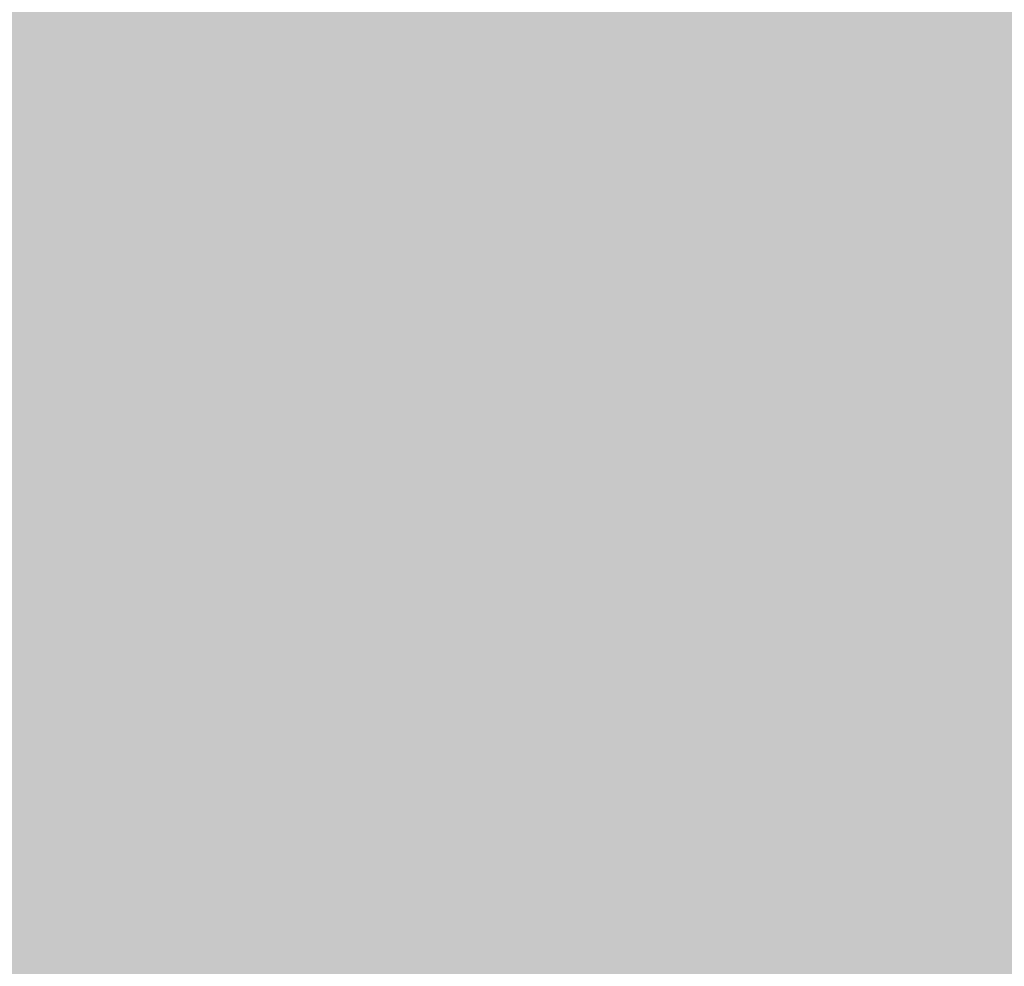
# Model space of a CAD drawing. Units: inches. Extents: x 2083 to 3317, y 1141 to 2115.
# Tile 132 of 256: x 3119.674 to 3123.979, y 1267.234 to 1271.372. Entities that reach past the tile are written whole.
import ezdxf

# ---------------------------------------------------------------- set-up
doc = ezdxf.new("R2010")
doc.units = ezdxf.units.IN
doc.layers.add('A-ANNO-DIMS', color=2, linetype='Continuous', lineweight=18)
doc.layers.add('A-WALL-PATT', color=251, linetype='Continuous', lineweight=13, true_color=0x636466)
doc.styles.get("Standard").update_dxf_attribs({"font": 'arial.ttf'})
doc.dimstyles.new('ISO-25', dxfattribs={"dimtxt": 12, "dimasz": 12, "dimexe": 1.25, "dimexo": 0.625, "dimtad": 1, "dimlunit": 3, "dimtxsty": 'Standard', "dimcen": 2.5, "dimadec": 0, "dimazin": 0, "dimtfac": 1, "dimtmove": 0, "dimatfit": 3, "dimfxl": 1, "dimarcsym": 0})

# ---------------------------------------------------------------- blocks, each defined once
blk = doc.blocks.new('*D26')
at = {"layer": 'A-ANNO-DIMS', "color": 0, "lineweight": -2, "transparency": 16777216}
for p, q in [((3088.9858, 1274.9151), (3088.9858, 1270.952)), ((3111.24, 1274.9151), (3111.24, 1270.952)), ((3076.9858, 1272.202), (2840.2624, 1272.202)), ((3111.24, 1272.202), (3088.9858, 1272.202)), ((3123.24, 1272.202), (3135.24, 1272.202))]:
    blk.add_line(p, q, dxfattribs=at)
at = {"layer": 'A-ANNO-DIMS', "color": 0, "transparency": 16777216}
for points in [[(3076.9858, 1274.202), (3076.9858, 1270.202), (3088.9858, 1272.202)], [(3123.24, 1274.202), (3123.24, 1270.202), (3111.24, 1272.202)]]:
    blk.add_solid(points, dxfattribs=at)
at = {"layer": 'Defpoints', "color": 0, "transparency": 16777216}
for p in [(3088.9858, 1275.5401), (3111.24, 1275.5401), (3088.9858, 1272.202)]:
    blk.add_point(p, dxfattribs=at)
at = {"layer": 'A-ANNO-DIMS', "color": 0, "transparency": 16777216, "insert": (2952.6241, 1279.0316), "char_height": 12, "attachment_point": 5}
blk.add_mtext('NIGHTSTAND 1\'-10 1/2" TYP.', dxfattribs=at)
blk = doc.blocks.new('*D27')
at = {"layer": 'A-ANNO-DIMS', "color": 0, "lineweight": -2, "transparency": 16777216}
for p, q in [((3114.5782, 1309.7943), (3114.5782, 1321.7943)), ((3111.865, 1297.7943), (3115.8282, 1297.7943)), ((3114.5782, 1297.7943), (3114.5782, 1275.5401)), ((3111.865, 1275.5401), (3115.8282, 1275.5401)), ((3114.5782, 1263.5401), (3114.5782, 1140.9886))]:
    blk.add_line(p, q, dxfattribs=at)
at = {"layer": 'A-ANNO-DIMS', "color": 0, "transparency": 16777216}
for points in [[(3112.5782, 1309.7943), (3116.5782, 1309.7943), (3114.5782, 1297.7943)], [(3112.5782, 1263.5401), (3116.5782, 1263.5401), (3114.5782, 1275.5401)]]:
    blk.add_solid(points, dxfattribs=at)
at = {"layer": 'Defpoints', "color": 0, "transparency": 16777216}
for p in [(3111.24, 1297.7943), (3111.24, 1275.5401), (3114.5782, 1275.5401)]:
    blk.add_point(p, dxfattribs=at)
at = {"layer": 'A-ANNO-DIMS', "color": 0, "transparency": 16777216, "insert": (3107.7485, 1196.2643), "char_height": 12, "attachment_point": 5, "rotation": 90}
blk.add_mtext('1\'-10 1/2" TYP.', dxfattribs=at)

msp = doc.modelspace()

# ---------------------------------------------------------------- hatches: boundary and pattern name
at = {"layer": 'A-WALL-PATT'}
h = msp.add_hatch(color=256, dxfattribs=at)
h.dxf.hatch_style = 1
h.paths.add_polyline_path([(3126.9598, 2020.7614), (2748.9598, 2020.7614), (2604.9598, 2020.7614), (2226.9598, 2020.7614), (2226.9598, 1702.7614), (2466.9598, 1702.7614), (2466.9598, 1582.7614), (2418.9598, 1582.7614), (2418.9598, 1477.7614), (2226.9598, 1477.7614), (2226.9598, 1263.2614), (2544.9598, 1263.2614), (2544.9598, 1411.7614), (2604.9598, 1411.7614), (2685.9598, 1411.7614), (2685.9598, 1420.7614), (2604.9598, 1420.7614), (2604.9598, 1573.7614), (2604.9598, 1702.7614), (2604.9598, 2011.7614), (2748.9598, 2011.7614), (2748.9598, 1702.7614), (2862.9598, 1702.7614), (2862.9598, 1621.7614), (2871.9598, 1621.7614), (2871.9598, 1702.7614), (2883.9598, 1702.7614), (2883.9598, 1706.9395, -0.026459), (2883.9598, 1711.7614), (2757.9598, 1711.7614), (2757.9598, 1807.7614), (2787.9598, 1807.7614), (2787.9598, 1812.2614), (2757.9598, 1812.2614), (2757.9598, 2011.7614), (2877.9598, 2011.7614), (2877.9598, 1812.2614), (2847.9598, 1812.2614), (2847.9598, 1807.7614), (2889.8357, 1807.7614), (2889.8357, 1812.2614), (2882.4598, 1812.2614), (2882.4598, 2011.7614), (3117.9598, 2011.7614), (3117.9598, 1812.2614), (2937.8357, 1812.2614), (2937.8357, 1807.7614), (2995.7098, 1807.7614), (2995.7098, 1796.1177), (3000.2098, 1796.1177), (3000.2098, 1807.7614), (3117.9598, 1807.7614), (3117.9598, 1711.7614), (3000.2098, 1711.7614), (3000.2098, 1760.1177), (2998.5727, 1760.1177, -0.020711), (2995.7098, 1760.1177), (2995.7098, 1711.7614), (2931.9598, 1711.7614), (2931.9598, 1702.7614), (3126.9598, 1702.7614)])
h.paths.add_polyline_path([(2471.4598, 2011.7614), (2471.4598, 1810.0114), (2462.7169, 1810.0114), (2462.7169, 1805.5114), (2505.9598, 1805.5114), (2505.9598, 1810.0114), (2475.9598, 1810.0114), (2475.9598, 2011.7614), (2595.9598, 2011.7614), (2595.9598, 1810.0114), (2565.9598, 1810.0114), (2565.9598, 1805.5114), (2595.9598, 1805.5114), (2595.9598, 1711.7614), (2235.9598, 1711.7614), (2235.9598, 1805.5114), (2353.7098, 1805.5114), (2353.7098, 1796.0542), (2358.2098, 1796.0542), (2358.2098, 1805.5114), (2414.7169, 1805.5114), (2414.7169, 1810.0114), (2235.9598, 1810.0114), (2235.9598, 2011.7614)], flags=16)
h.paths.add_polyline_path([(2270.2047, 1994.61), (2270.2047, 1970.61), (2246.2047, 1970.61), (2246.2047, 1994.61)], flags=0)
edge = h.paths.add_edge_path(flags=0)
edge.add_ellipse((2332.0274, 1899.7982), major_axis=(-3.043, 3.043), ratio=0.168252, start_angle=-161.3322, end_angle=-156.3071, ccw=False)
edge.add_ellipse((2333.082, 1898.7435), major_axis=(-1.0546, 1.0546), ratio=0.453532, start_angle=-123.371, end_angle=-94.1591)
edge = h.paths.add_edge_path(flags=0)
edge.add_ellipse((2332.0274, 1968.8763), major_axis=(3.043, 3.043), ratio=0.168252, start_angle=18.6678, end_angle=23.6929)
edge.add_spline(control_points=[(2332.9256, 1970.6911), (2332.2268, 1970.3361), (2330.8937, 1969.6589), (2328.4131, 1970.9321), (2327.2039, 1967.7487), (2324.7096, 1969.9556), (2322.5328, 1967.0124), (2320.0128, 1971.2958), (2317.6803, 1968.1578), (2316.0405, 1967.102), (2315.4269, 1966.8096)], knot_values=[0, 0, 0, 0, 2.267059, 4.324559, 6.685584, 8.878641, 11.121502, 14.300359, 17.755284, 19.732645, 19.732645, 19.732645, 19.732645], degree=3, periodic=0)
edge.add_ellipse((2332.0274, 1968.8763), major_axis=(3.043, 3.043), ratio=0.168252, start_angle=18.6678, end_angle=23.6929, ccw=False)
edge.add_ellipse((2333.082, 1969.9309), major_axis=(1.0546, 1.0546), ratio=0.453532, start_angle=56.629, end_angle=85.8409, ccw=False)
edge = h.paths.add_edge_path(flags=0)
edge.add_spline(control_points=[(2296.4283, 1967.9879), (2293.6278, 1965.3363), (2287.7036, 1959.7271), (2299.7439, 1949.9957), (2294.5326, 1935.6685), (2290.5732, 1920.6035), (2293.3941, 1909.9737), (2296.1854, 1904.9665)], knot_values=[0.099185, 0.099185, 0.099185, 0.099185, 0.345301, 0.619822, 0.982653, 1.386093, 1.810555, 1.810555, 1.810555, 1.810555], degree=3, periodic=0)
edge.add_spline(control_points=[(2296.1854, 1904.9665), (2297.3836, 1902.6193), (2298.001, 1901.9493), (2298.553, 1901.4682)], knot_values=[0.006246, 0.006246, 0.006246, 0.006246, 0.055476, 0.055476, 0.055476, 0.055476], degree=3, periodic=0)
edge.add_spline(control_points=[(2298.553, 1901.4682), (2297.2586, 1900.9232), (2295.2253, 1900.2321), (2293.0602, 1900.6142), (2292.1014, 1900.7884), (2292.0896, 1900.7906)], knot_values=[0.312835, 0.312835, 0.312835, 0.312835, 0.40178, 0.474987, 0.475903, 0.475903, 0.475903, 0.475903], degree=3, periodic=0)
edge.add_arc((2292.7936, 1904.6641), 3.937, 215.4209, 259.6982, ccw=False)
edge.add_spline(control_points=[(2289.5853, 1902.3823), (2289.4767, 1902.5351), (2289.3685, 1902.688), (2289.2609, 1902.8412)], knot_values=[0.102872, 0.102872, 0.102872, 0.102872, 0.116896, 0.116896, 0.116896, 0.116896], degree=3, periodic=0)
edge.add_spline(control_points=[(2289.2609, 1902.8412), (2288.6866, 1902.5502), (2287.64, 1902.0199), (2285.8813, 1901.874), (2283.853, 1901.5044), (2281.72, 1899.7105), (2278.467, 1899.4929), (2276.1571, 1901.8832), (2272.259, 1899.8041), (2267.7776, 1901.8432), (2262.2439, 1900.184), (2257.4149, 1901.7821), (2254.3184, 1900.7261), (2253.1783, 1900.3373)], knot_values=[0, 0, 0, 0, 1.907977, 3.477176, 5.261074, 7.972851, 11.680248, 13.717921, 16.939592, 22.789562, 27.502503, 33.595215, 37.145618, 37.145618, 37.145618, 37.145618], degree=3, periodic=0)
edge.add_line((2253.1783, 1900.3373), (2250.2442, 1902.8412))
edge.add_line((2250.2442, 1902.8412), (2250.2442, 1965.8333))
edge.add_line((2250.2442, 1965.8333), (2253.1783, 1968.3371))
edge.add_spline(control_points=[(2253.1783, 1968.3371), (2254.3184, 1967.9483), (2257.4149, 1966.8924), (2262.2439, 1968.4904), (2267.7776, 1966.8313), (2271.5267, 1968.5372), (2273.8759, 1967.8283), (2274.2067, 1967.7276)], knot_values=[0, 0, 0, 0, 0.09018, 0.244935, 0.364644, 0.513233, 0.537855, 0.537855, 0.537855, 0.537855], degree=3, periodic=0)
edge.add_arc((2274.3529, 1963.7933), 3.937, 72.0511, 92.1279, ccw=False)
edge.add_arc((2281.2969, 1985.23), 18.5963, 252.05113, 288.56572)
edge.add_arc((2292.3167, 1956.0289), 12.6461, 71.02679, 113.77822, ccw=False)
edge = h.paths.add_edge_path(flags=0)
edge.add_spline(control_points=[(2274.8994, 1951.8562), (2275.0662, 1951.6166), (2275.2327, 1951.3766), (2275.398, 1951.1359)], knot_values=[1.409916, 1.409916, 1.409916, 1.409916, 1.43159, 1.43159, 1.43159, 1.43159], degree=3, periodic=0)
edge.add_spline(control_points=[(2275.398, 1951.1359), (2275.7921, 1950.5619), (2276.1792, 1949.9838), (2276.5455, 1949.3971)], knot_values=[1.358238, 1.358238, 1.358238, 1.358238, 1.409916, 1.409916, 1.409916, 1.409916], degree=3, periodic=0)
edge.add_line((2276.5455, 1949.3971), (2277.4373, 1947.8622))
edge.add_spline(control_points=[(2277.4373, 1947.8622), (2276.3038, 1945.6731), (2274.6397, 1942.4269), (2274.6316, 1938.0939), (2272.7991, 1930.8515), (2274.3564, 1943.897), (2275.9477, 1947.9234), (2276.5455, 1949.3971)], knot_values=[0.005632, 0.005632, 0.005632, 0.005632, 0.186014, 0.266002, 0.357087, 0.59639, 0.739732, 0.739732, 0.739732, 0.739732], degree=3, periodic=0)
edge.add_spline(control_points=[(2276.5455, 1949.3971), (2276.1792, 1949.9838), (2275.7921, 1950.5619), (2275.398, 1951.1359)], knot_values=[1.358238, 1.358238, 1.358238, 1.358238, 1.409916, 1.409916, 1.409916, 1.409916], degree=3, periodic=0)
edge.add_spline(control_points=[(2275.398, 1951.1359), (2274.9425, 1950.0805), (2274.2078, 1948.0253), (2273.9346, 1944.8515), (2272.4685, 1937.6275), (2273.4662, 1945.6965), (2274.7006, 1951.0595), (2274.8994, 1951.8562)], knot_values=[0.104364, 0.104364, 0.104364, 0.104364, 0.189636, 0.269624, 0.36071, 0.600013, 0.644622, 0.644622, 0.644622, 0.644622], degree=3, periodic=0)
h.paths.add_polyline_path([(2269.1675, 1963.1276, -0.357527), (2268.1706, 1960.9764, -0.092561), (2268.1706, 1939.4363, -0.357527), (2269.1675, 1937.2851, -0.357527), (2267.0163, 1938.282, -0.164785), (2254.6856, 1938.282, -0.357527), (2252.5344, 1937.2851, -0.357527), (2253.5313, 1939.4363, -0.092561), (2253.5313, 1960.9764, -0.357527), (2252.5344, 1963.1276, -0.357527), (2254.6856, 1962.1307, -0.164785), (2267.0163, 1962.1307, -0.357527)], flags=0)
h.paths.add_polyline_path([(2248.8741, 1967.8018), (2248.8741, 1957.0277), (2249.4578, 1957.0277), (2249.4578, 1911.6468), (2248.8741, 1911.6468), (2248.8741, 1900.8727), (2246.5119, 1900.8727, 0.197327), (2244.1497, 1902.4569), (2244.1497, 1966.2176, 0.197327), (2246.5119, 1967.8018)], flags=0)
h.paths.add_polyline_path([(2269.1675, 1931.3893, -0.357527), (2268.1706, 1929.2381, -0.092561), (2268.1706, 1907.6981, -0.357527), (2269.1675, 1905.5469, -0.357527), (2267.0163, 1906.5438, -0.164785), (2254.6856, 1906.5438, -0.357527), (2252.5344, 1905.5469, -0.357527), (2253.5313, 1907.6981, -0.092561), (2253.5313, 1929.2381, -0.357527), (2252.5344, 1931.3893, -0.357527), (2254.6856, 1930.3925, -0.164785), (2267.0163, 1930.3925, -0.357527)], flags=0)
edge = h.paths.add_edge_path(flags=0)
edge.add_spline(control_points=[(2276.1969, 1906.7237), (2276.1681, 1909.0289), (2276.114, 1913.3719), (2270.5984, 1924.925), (2273.9052, 1919.0128), (2275.9217, 1916.2621), (2275.4746, 1912.4021), (2277.2579, 1910.3806), (2276.696, 1908.225), (2276.6462, 1906.813), (2276.6178, 1906.0084)], knot_values=[0, 0, 0, 0, 8.61026, 16.221274, 18.843057, 23.804898, 27.440828, 29.356102, 31.203478, 33.650687, 33.650687, 33.650687, 33.650687], degree=3, periodic=0)
edge.add_spline(control_points=[(2276.6178, 1906.0084), (2276.6233, 1905.6241), (2276.4977, 1904.6287), (2275.4418, 1903.8547), (2274.9373, 1903.0804), (2274.8591, 1902.8412)], knot_values=[0.156488, 0.156488, 0.156488, 0.156488, 0.184398, 0.231376, 0.250598, 0.250598, 0.250598, 0.250598], degree=3, periodic=0)
edge.add_line((2274.8591, 1902.8412), (2276.506, 1902.8412))
edge.add_spline(control_points=[(2276.506, 1902.8412), (2276.7883, 1903.0849), (2277.6651, 1904.1252), (2278.2495, 1904.3407), (2277.6539, 1908.5274), (2278.1557, 1906.2278), (2278.1005, 1905.2859), (2278.8467, 1904.069), (2277.8568, 1903.4149), (2277.8742, 1902.991), (2277.9036, 1902.8412)], knot_values=[0.059574, 0.059574, 0.059574, 0.059574, 0.080753, 0.103741, 0.16972, 0.176036, 0.207137, 0.240474, 0.262341, 0.27366, 0.27366, 0.27366, 0.27366], degree=3, periodic=0)
edge.add_line((2277.9036, 1902.8412), (2280.0298, 1902.8412))
edge.add_spline(control_points=[(2280.0298, 1902.8412), (2279.8882, 1903.0884), (2279.4993, 1903.9816), (2280.1523, 1905.9393), (2278.1036, 1909.6578), (2279.7624, 1907.1853), (2280.3279, 1904.8749), (2280.4851, 1903.4896), (2281.4633, 1903.2494), (2281.7583, 1902.9365), (2281.834, 1902.8412)], knot_values=[0.013856, 0.013856, 0.013856, 0.013856, 0.034874, 0.088867, 0.107879, 0.126738, 0.158714, 0.193757, 0.217487, 0.226722, 0.226722, 0.226722, 0.226722], degree=3, periodic=0)
edge.add_spline(control_points=[(2281.834, 1902.8412), (2281.7875, 1902.8267), (2281.647, 1902.783), (2281.3955, 1902.8595), (2281.0881, 1902.9852), (2280.7207, 1903.0609), (2280.3335, 1903.0257), (2280.1248, 1902.8989), (2280.0298, 1902.8412)], knot_values=[0, 0, 0, 0, 0.14413, 0.435517, 0.749276, 1.153046, 1.548371, 1.878348, 1.878348, 1.878348, 1.878348], degree=3, periodic=0)
edge.add_line((2280.0298, 1902.8412), (2277.9036, 1902.8412))
edge.add_spline(control_points=[(2277.9036, 1902.8412), (2277.8929, 1902.7959), (2277.8654, 1902.6796), (2277.6075, 1902.6875), (2277.2741, 1902.8007), (2276.8379, 1902.6198), (2276.5838, 1902.7893), (2276.506, 1902.8412)], knot_values=[0, 0, 0, 0, 0.127189, 0.326199, 0.628009, 1.24357, 1.515331, 1.515331, 1.515331, 1.515331], degree=3, periodic=0)
edge.add_line((2276.506, 1902.8412), (2274.8591, 1902.8412))
edge.add_spline(control_points=[(2274.8591, 1902.8412), (2274.8144, 1902.8986), (2274.7251, 1903.0134), (2274.4935, 1903.119), (2274.2443, 1902.9605), (2273.9371, 1903.1849), (2273.614, 1902.9831), (2273.4083, 1902.883), (2273.3223, 1902.8412)], knot_values=[0, 0, 0, 0, 0.21843, 0.436957, 0.687977, 0.990379, 1.398396, 1.69185, 1.69185, 1.69185, 1.69185], degree=3, periodic=0)
edge.add_spline(control_points=[(2273.3223, 1902.8412), (2273.6167, 1903.4457), (2274.274, 1904.5383), (2276.0272, 1904.5737), (2276.207, 1906.5836), (2276.1969, 1906.7237)], knot_values=[0.012227, 0.012227, 0.012227, 0.012227, 0.059472, 0.106218, 0.134458, 0.134458, 0.134458, 0.134458], degree=3, periodic=0)
h.paths.add_polyline_path([(2270.7761, 1897.7898), (2270.7761, 1873.7898), (2246.7761, 1873.7898), (2246.7761, 1897.7898)], flags=0)
h.paths.add_polyline_path([(2353.7098, 1760.0051), (2353.7098, 1760.0542), (2358.2098, 1760.0542, -0.033729)], flags=0)
h.paths.add_polyline_path([(2321.8191, 1737.5292), (2341.9953, 1737.5292, -0.414214), (2343.2033, 1736.3212), (2343.2033, 1721.0206, -0.414214), (2341.9953, 1719.8127), (2321.8191, 1719.8127, -0.414214), (2320.6112, 1721.0206), (2320.6112, 1736.3212, -0.414214)], flags=0)
h.paths.add_polyline_path([(2324.235, 1736.3212), (2339.5794, 1736.3212, -0.414214), (2341.9953, 1733.9053), (2341.9953, 1725.4497, -0.414214), (2339.5794, 1723.0338), (2333.6806, 1723.0338), (2333.8453, 1722.0455, -0.870646), (2335.4254, 1721.8259, -0.767327), (2333.9227, 1721.4232), (2331.291, 1721.4232, -0.767327), (2329.7883, 1721.8259, -0.870646), (2331.3684, 1722.0455), (2331.5331, 1723.0338), (2324.235, 1723.0338, -0.414214), (2321.8191, 1725.4497), (2321.8191, 1733.9053, -0.414214)], flags=0)
h.paths.add_polyline_path([(2570.4838, 1928.6154), (2589.6838, 1928.6154), (2590.1688, 1928.6154), (2590.1688, 1904.9934), (2570.4838, 1904.9934)], flags=0)
h.paths.add_polyline_path([(2574.4473, 1927.2638, -1), (2572.8288, 1927.2638, -1)], flags=0)
h.paths.add_polyline_path([(2573.0899, 1926.9409), (2573.925, 1927.776), (2574.1477, 1927.5533), (2573.3126, 1926.7182)], flags=0)
h.paths.add_polyline_path([(2578.7791, 1919.7296, -1), (2571.5917, 1919.7296, -1)], flags=0)
h.paths.add_polyline_path([(2578.3854, 1919.7296, -1), (2571.9854, 1919.7296, -1)], flags=0)
h.paths.add_polyline_path([(2331.5958, 1729.4762, -1), (2333.618, 1729.4762, -1)], flags=0)
h.paths.add_polyline_path([(2578.0342, 1927.2638, -1), (2576.4157, 1927.2638, -1)], flags=0)
h.paths.add_polyline_path([(2576.6889, 1927.5311), (2576.9116, 1927.7538), (2577.7467, 1926.9186), (2577.524, 1926.6959)], flags=0)
h.paths.add_polyline_path([(2578.1391, 1909.8595, -1), (2572.2317, 1909.8595, -1)], flags=0)
h.paths.add_polyline_path([(2577.7454, 1909.8595, -1), (2572.6254, 1909.8595, -1)], flags=0)
h.paths.add_polyline_path([(2583.7977, 1927.2638, -1), (2582.1792, 1927.2638, -1)], flags=0)
h.paths.add_polyline_path([(2582.7186, 1927.7538), (2583.5538, 1926.9186), (2583.3311, 1926.6959), (2582.4959, 1927.5311)], flags=0)
h.paths.add_polyline_path([(2582.4959, 1927.5311), (2582.7186, 1927.7538), (2583.5538, 1926.9186), (2583.3311, 1926.6959)], flags=0)
h.paths.add_polyline_path([(2587.7391, 1920.5296, -1), (2581.8317, 1920.5296, -1)], flags=0)
h.paths.add_polyline_path([(2587.3454, 1920.5296, -1), (2582.2254, 1920.5296, -1)], flags=0)
h.paths.add_polyline_path([(2587.3846, 1927.2638, -1), (2585.7661, 1927.2638, -1)], flags=0)
h.paths.add_polyline_path([(2586.082, 1926.9802), (2586.9172, 1927.8154), (2587.1399, 1927.5927), (2586.3047, 1926.7575)], flags=0)
h.paths.add_polyline_path([(2588.3791, 1910.6595, -1), (2581.1917, 1910.6595, -1)], flags=0)
h.paths.add_polyline_path([(2587.9854, 1910.6595, -1), (2581.5854, 1910.6595, -1)], flags=0)
h.paths.add_polyline_path([(2417.1677, 1729.4779), (2437.3439, 1729.4779, -0.414214), (2438.5519, 1728.2699), (2438.5519, 1712.9693, -0.414214), (2437.3439, 1711.7614), (2417.1677, 1711.7614, -0.414214), (2415.9598, 1712.9693), (2415.9598, 1728.2699, -0.414214)], flags=0)
h.paths.add_polyline_path([(2419.5836, 1728.2699), (2434.928, 1728.2699, -0.414214), (2437.3439, 1725.8541), (2437.3439, 1717.3984, -0.414214), (2434.928, 1714.9825), (2429.0292, 1714.9825), (2429.1939, 1713.9942, -0.870646), (2430.774, 1713.7746, -0.767327), (2429.2713, 1713.372), (2426.6396, 1713.372, -0.767327), (2425.1369, 1713.7746, -0.870646), (2426.717, 1713.9942), (2426.8817, 1714.9825), (2419.5836, 1714.9825, -0.414214), (2417.1677, 1717.3984), (2417.1677, 1725.8541, -0.414214)], flags=0)
h.paths.add_polyline_path([(2419.5836, 1728.2699), (2434.928, 1728.2699, -0.414214), (2437.3439, 1725.8541), (2437.3439, 1717.3984, -0.414214), (2434.928, 1714.9825), (2429.0292, 1714.9825), (2428.3581, 1719.009), (2427.5528, 1719.009), (2426.8817, 1714.9825), (2419.5836, 1714.9825, -0.414214), (2417.1677, 1717.3984), (2417.1677, 1725.8541, -0.414214)], flags=0)
h.paths.add_polyline_path([(2426.9444, 1721.4249, -1), (2428.9666, 1721.4249, -1)], flags=0)
h.paths.add_polyline_path([(2475.9598, 1702.7614), (2595.9598, 1702.7614), (2595.9598, 1582.7614), (2475.9598, 1582.7614)], flags=16)
h.paths.add_polyline_path([(2427.9598, 1573.7614), (2595.9598, 1573.7614), (2595.9598, 1468.7614), (2595.9598, 1420.7614), (2384.4598, 1420.7614), (2384.4598, 1468.7614), (2427.9598, 1468.7614)], flags=16)
h.paths.add_polyline_path([(2379.9598, 1468.7614), (2379.9598, 1420.7614), (2235.9598, 1420.7614), (2235.9598, 1468.7614)], flags=16)
h.paths.add_polyline_path([(2317.816, 1466.6958), (2337.9922, 1466.6958, -0.414214), (2339.2002, 1465.4878), (2339.2002, 1450.1872, -0.414214), (2337.9922, 1448.9792), (2317.816, 1448.9792, -0.414214), (2316.6081, 1450.1872), (2316.6081, 1465.4878, -0.414214)], flags=0)
h.paths.add_polyline_path([(2320.2319, 1465.4878), (2335.5763, 1465.4878, -0.414214), (2337.9922, 1463.0719), (2337.9922, 1454.6163, -0.414214), (2335.5763, 1452.2004), (2329.6775, 1452.2004), (2329.8422, 1451.212, -0.870646), (2331.4223, 1450.9925, -0.767327), (2329.9196, 1450.5898), (2327.2879, 1450.5898, -0.767327), (2325.7852, 1450.9925, -0.870646), (2327.3653, 1451.212), (2327.53, 1452.2004), (2320.2319, 1452.2004, -0.414214), (2317.816, 1454.6163), (2317.816, 1463.0719, -0.414214)], flags=0)
h.paths.add_polyline_path([(2320.2319, 1465.4878), (2335.5763, 1465.4878, -0.414214), (2337.9922, 1463.0719), (2337.9922, 1454.6163, -0.414214), (2335.5763, 1452.2004), (2329.6775, 1452.2004), (2329.0064, 1456.2269), (2328.2011, 1456.2269), (2327.53, 1452.2004), (2320.2319, 1452.2004, -0.414214), (2317.816, 1454.6163), (2317.816, 1463.0719, -0.414214)], flags=0)
h.paths.add_polyline_path([(2327.5926, 1458.6428, -1), (2329.6148, 1458.6428, -1)], flags=0)
h.paths.add_polyline_path([(2244.4117, 1433.3405), (2241.9209, 1433.3405, -0.414214), (2240.0179, 1435.2435), (2240.0179, 1440.9528, -0.414211), (2241.9209, 1442.8559), (2244.4117, 1442.8559, -1.976472)], flags=0)
h.paths.add_polyline_path([(2245.3569, 1434.3975, -0.414214), (2245.3569, 1441.7988, -2.144098)], flags=0)
h.paths.add_polyline_path([(2535.9598, 1416.2614), (2535.9598, 1272.2614), (2235.9598, 1272.2614), (2235.9598, 1416.2614)], flags=16)
h.paths.add_polyline_path([(2260.1196, 1384.2928), (2260.1196, 1362.0386), (2237.8654, 1362.0386), (2237.8654, 1384.2928)], flags=0)
edge = h.paths.add_edge_path(flags=0)
edge.add_line((2318.2518, 1362.0933), (2318.1458, 1362.001))
edge.add_ellipse((2317.4451, 1360.431), major_axis=(2.8216, 2.8216), ratio=0.168252, start_angle=18.6678, end_angle=20.9481, ccw=False)
edge.add_ellipse((2318.423, 1361.409), major_axis=(0.9779, 0.9779), ratio=0.453532, start_angle=56.629, end_angle=70.2262, ccw=False)
edge = h.paths.add_edge_path(flags=0)
edge.add_line((2319.1074, 1295.5711), (2319.015, 1295.6771))
edge.add_ellipse((2317.4451, 1296.3778), major_axis=(-2.8216, 2.8216), ratio=0.168252, start_angle=-161.3322, end_angle=-159.0519, ccw=False)
edge.add_ellipse((2318.423, 1295.3999), major_axis=(-0.9779, 0.9779), ratio=0.453532, start_angle=-123.371, end_angle=-109.7738)
edge = h.paths.add_edge_path(flags=0)
edge.add_spline(control_points=[(2284.2103, 1301.1702), (2284.5807, 1300.4447), (2284.8912, 1299.892), (2285.1596, 1299.461)], knot_values=[0.039066, 0.039066, 0.039066, 0.039066, 0.055476, 0.055476, 0.055476, 0.055476], degree=3, periodic=0)
edge.add_line((2285.1596, 1299.461), (2284.2103, 1301.1702))
edge = h.paths.add_edge_path(flags=0)
edge.add_line((2280.4125, 1297.298), (2283.37, 1297.0361))
edge.add_line((2283.37, 1297.0361), (2286.4057, 1297.9263))
edge.add_spline(control_points=[(2286.4057, 1297.9263), (2285.3055, 1297.4631), (2284.3448, 1297.1292), (2283.37, 1297.0361)], knot_values=[0.394369, 0.394369, 0.394369, 0.394369, 0.475903, 0.475903, 0.475903, 0.475903], degree=3, periodic=0)
edge.add_spline(control_points=[(2283.37, 1297.0361), (2283.2814, 1297.0277), (2282.3163, 1296.9573), (2281.3125, 1297.1345), (2280.4234, 1297.296), (2280.4125, 1297.298)], knot_values=[0.312835, 0.312835, 0.312835, 0.312835, 0.320246, 0.393453, 0.394369, 0.394369, 0.394369, 0.394369], degree=3, periodic=0)
edge = h.paths.add_edge_path(flags=0)
edge.add_line((2284.4356, 1359.6073), (2280.4463, 1355.328))
edge.add_line((2280.4463, 1355.328), (2279.58, 1351.0178))
edge.add_line((2279.58, 1351.0178), (2282.413, 1346.5804))
edge.add_spline(control_points=[(2282.413, 1346.5804), (2283.1533, 1345.5892), (2284.2529, 1344.0289), (2284.801, 1342.3872), (2284.9352, 1341.8055)], knot_values=[1.240098, 1.240098, 1.240098, 1.240098, 1.332892, 1.382712, 1.382712, 1.382712, 1.382712], degree=3, periodic=0)
edge.add_spline(control_points=[(2284.9352, 1341.8055), (2285.3191, 1340.1406), (2285.233, 1338.4092), (2284.9099, 1336.6541)], knot_values=[1.097484, 1.097484, 1.097484, 1.097484, 1.240098, 1.240098, 1.240098, 1.240098], degree=3, periodic=0)
edge.add_spline(control_points=[(2284.9099, 1336.6541), (2284.5868, 1334.899), (2284.0267, 1333.1203), (2283.4626, 1331.3606)], knot_values=[0.95487, 0.95487, 0.95487, 0.95487, 1.097484, 1.097484, 1.097484, 1.097484], degree=3, periodic=0)
edge.add_line((2283.4626, 1331.3606), (2281.8904, 1326.1534))
edge.add_line((2281.8904, 1326.1534), (2280.7563, 1321.0561))
edge.add_line((2280.7563, 1321.0561), (2280.2992, 1316.002))
edge.add_line((2280.2992, 1316.002), (2280.7159, 1310.9501))
edge.add_line((2280.7159, 1310.9501), (2282.0281, 1305.9721))
edge.add_line((2282.0281, 1305.9721), (2284.2103, 1301.1702))
edge.add_spline(control_points=[(2284.2103, 1301.1702), (2283.3407, 1302.7302), (2282.6119, 1304.3365), (2282.0281, 1305.9721)], knot_values=[0.099185, 0.099185, 0.099185, 0.099185, 0.241799, 0.241799, 0.241799, 0.241799], degree=3, periodic=0)
edge.add_spline(control_points=[(2282.0281, 1305.9721), (2281.4443, 1307.6078), (2281.0055, 1309.2728), (2280.7159, 1310.9501)], knot_values=[0.241799, 0.241799, 0.241799, 0.241799, 0.384413, 0.384413, 0.384413, 0.384413], degree=3, periodic=0)
edge.add_spline(control_points=[(2280.7159, 1310.9501), (2280.4332, 1312.5876), (2280.2894, 1314.277), (2280.2989, 1315.962), (2280.2992, 1316.002)], knot_values=[0.384413, 0.384413, 0.384413, 0.384413, 0.523647, 0.527028, 0.527028, 0.527028, 0.527028], degree=3, periodic=0)
edge.add_spline(control_points=[(2280.2992, 1316.002), (2280.3123, 1317.687), (2280.4779, 1319.3679), (2280.7563, 1321.0561)], knot_values=[0.527028, 0.527028, 0.527028, 0.527028, 0.669642, 0.669642, 0.669642, 0.669642], degree=3, periodic=0)
edge.add_spline(control_points=[(2280.7563, 1321.0561), (2281.0346, 1322.7443), (2281.4259, 1324.4396), (2281.8904, 1326.1534)], knot_values=[0.669642, 0.669642, 0.669642, 0.669642, 0.812256, 0.812256, 0.812256, 0.812256], degree=3, periodic=0)
edge.add_spline(control_points=[(2281.8904, 1326.1534), (2282.2644, 1327.5333), (2282.7879, 1329.2618), (2283.3528, 1331.0178), (2283.4626, 1331.3606)], knot_values=[0.812256, 0.812256, 0.812256, 0.812256, 0.927087, 0.95487, 0.95487, 0.95487, 0.95487], degree=3, periodic=0)
edge.add_line((2283.4626, 1331.3606), (2284.9099, 1336.6541))
edge.add_line((2284.9099, 1336.6541), (2284.9352, 1341.8055))
edge.add_line((2284.9352, 1341.8055), (2282.413, 1346.5804))
edge.add_spline(control_points=[(2282.413, 1346.5804), (2281.2751, 1348.1038), (2280.0784, 1349.5703), (2279.58, 1351.0178)], knot_values=[1.382712, 1.382712, 1.382712, 1.382712, 1.525326, 1.525326, 1.525326, 1.525326], degree=3, periodic=0)
edge.add_spline(control_points=[(2279.58, 1351.0178), (2279.4433, 1351.4147), (2279.1363, 1352.8569), (2279.7352, 1354.2904), (2280.4463, 1355.328)], knot_values=[1.525326, 1.525326, 1.525326, 1.525326, 1.564439, 1.667941, 1.667941, 1.667941, 1.667941], degree=3, periodic=0)
edge.add_spline(control_points=[(2280.4463, 1355.328), (2281.4261, 1356.7578), (2282.9308, 1358.1826), (2284.4356, 1359.6073)], knot_values=[1.667941, 1.667941, 1.667941, 1.667941, 1.810555, 1.810555, 1.810555, 1.810555], degree=3, periodic=0)
edge.add_arc((2280.6231, 1348.5182), 11.7262, 71.02679, 113.77822)
edge.add_arc((2270.4049, 1375.5952), 17.2436, 252.05113, 288.56572, ccw=False)
edge.add_arc((2263.966, 1355.7178), 3.6506, 72.0511, 92.1279)
edge.add_arc((2263.966, 1355.7178), 3.6506, 92.1279, 177.9851)
edge.add_spline(control_points=[(2260.3176, 1355.8462), (2260.2604, 1354.2207), (2260.5513, 1350.1865), (2262.9993, 1346.7663), (2264.4727, 1344.649)], knot_values=[1.43159, 1.43159, 1.43159, 1.43159, 1.564144, 1.770695, 1.770695, 1.770695, 1.770695], degree=3, periodic=0)
edge.add_line((2264.4727, 1344.649), (2264.9356, 1343.9825))
edge.add_spline(control_points=[(2263.801, 1340.2481), (2263.8432, 1340.5141), (2264.0672, 1341.7565), (2264.5127, 1343.0025), (2264.935, 1343.9811)], knot_values=[0.53657, 0.53657, 0.53657, 0.53657, 0.559349, 0.644622, 0.644622, 0.644622, 0.644622], degree=3, periodic=0)
edge.add_spline(control_points=[(2264.935, 1343.9811), (2265.1178, 1343.715), (2265.2989, 1343.4479), (2265.4768, 1343.1794)], knot_values=[1.384077, 1.384077, 1.384077, 1.384077, 1.409916, 1.409916, 1.409916, 1.409916], degree=3, periodic=0)
edge.add_spline(control_points=[(2265.4768, 1343.1794), (2265.6546, 1342.9108), (2265.8293, 1342.6408), (2265.9991, 1342.3688)], knot_values=[1.358238, 1.358238, 1.358238, 1.358238, 1.384077, 1.384077, 1.384077, 1.384077], degree=3, periodic=0)
edge.add_line((2265.9991, 1342.3688), (2266.826, 1340.9455))
edge.add_spline(control_points=[(2266.826, 1340.9455), (2268.8944, 1337.0897), (2271.3982, 1325.843), (2270.5162, 1310.5686), (2275.9194, 1301.8606), (2277.7895, 1299.1994)], knot_values=[0.116896, 0.116896, 0.116896, 0.116896, 0.472987, 1.050969, 1.313793, 1.313793, 1.313793, 1.313793], degree=3, periodic=0)
edge.add_spline(control_points=[(2277.7895, 1299.1994), (2277.8394, 1299.1285), (2277.8894, 1299.0575), (2277.9396, 1298.9866)], knot_values=[0.109884, 0.109884, 0.109884, 0.109884, 0.116896, 0.116896, 0.116896, 0.116896], degree=3, periodic=0)
edge.add_line((2277.9396, 1298.9866), (2277.7888, 1299.1991))
edge.add_spline(control_points=[(2277.7888, 1299.1991), (2277.2566, 1298.9294), (2276.2864, 1298.4379), (2275.0394, 1298.3344), (2274.3833, 1298.2389), (2274.2153, 1298.2093)], knot_values=[33.12187, 33.12187, 33.12187, 33.12187, 35.029056, 36.598255, 37.144827, 37.144827, 37.144827, 37.144827], degree=3, periodic=0)
edge.add_line((2274.2153, 1298.2093), (2273.0731, 1297.893))
edge.add_spline(control_points=[(2273.0731, 1297.893), (2272.3229, 1297.5798), (2271.0392, 1296.5105), (2269.2484, 1296.2261), (2268.4231, 1296.3747)], knot_values=[26.532584, 26.532584, 26.532584, 26.532584, 29.198919, 31.839101, 31.839101, 31.839101, 31.839101], degree=3, periodic=0)
edge.add_line((2268.4231, 1296.3747), (2263.8785, 1297.4575))
edge.add_spline(control_points=[(2263.8785, 1297.4575), (2263.5561, 1297.3594), (2261.8603, 1296.8387), (2260.2388, 1297.2824), (2258.9335, 1297.5165)], knot_values=[15.919551, 15.919551, 15.919551, 15.919551, 16.939592, 21.226067, 21.226067, 21.226067, 21.226067], degree=3, periodic=0)
edge.add_line((2258.9335, 1297.5165), (2254.0552, 1297.329))
edge.add_spline(control_points=[(2254.0552, 1297.329), (2253.7555, 1297.2958), (2252.1137, 1297.1652), (2250.4619, 1297.5442), (2249.1297, 1297.6679)], knot_values=[5.306517, 5.306517, 5.306517, 5.306517, 6.276435, 10.613034, 10.613034, 10.613034, 10.613034], degree=3, periodic=0)
edge.add_line((2249.1297, 1297.6679), (2244.3316, 1296.8778))
edge.add_line((2244.3316, 1296.8778), (2241.611, 1299.1994))
edge.add_line((2241.611, 1299.1994), (2241.611, 1357.6094))
edge.add_line((2241.611, 1357.6094), (2244.3316, 1359.9311))
edge.add_line((2244.3316, 1359.9311), (2252.7288, 1359.5427))
edge.add_spline(control_points=[(2252.7288, 1359.5427), (2252.8709, 1359.5464), (2253.3057, 1359.5482), (2253.7398, 1359.5143), (2254.0317, 1359.4824)], knot_values=[0.233291, 0.233291, 0.233291, 0.233291, 0.244935, 0.268927, 0.268927, 0.268927, 0.268927], degree=3, periodic=0)
edge.add_line((2254.0317, 1359.4824), (2259.5872, 1359.4164))
edge.add_spline(control_points=[(2259.5872, 1359.4164), (2260.6771, 1359.6285), (2262.0732, 1359.897), (2263.5237, 1359.4593), (2263.8304, 1359.366)], knot_values=[0.422516, 0.422516, 0.422516, 0.422516, 0.513233, 0.537855, 0.537855, 0.537855, 0.537855], degree=3, periodic=0)
edge.add_arc((2263.966, 1355.7178), 3.6506, 72.0511, 92.1279, ccw=False)
edge.add_arc((2270.4049, 1375.5952), 17.2436, 252.05113, 288.56572)
edge.add_arc((2280.6231, 1348.5182), 11.7262, 71.02679, 113.77822, ccw=False)
h.paths.add_polyline_path([(2240.3405, 1359.4347), (2240.3405, 1349.4444), (2240.8818, 1349.4444), (2240.8818, 1307.3645), (2240.3405, 1307.3645), (2240.3405, 1297.3741), (2238.1502, 1297.3741, 0.197327), (2235.9598, 1298.8431), (2235.9598, 1357.9657, 0.197327), (2238.1502, 1359.4347)], flags=0)
h.paths.add_polyline_path([(2259.1578, 1355.1005, -0.357527), (2258.2334, 1353.1058, -0.092561), (2258.2334, 1333.1326, -0.357527), (2259.1578, 1331.1379, -0.357527), (2257.1631, 1332.0622, -0.164785), (2245.7293, 1332.0622, -0.357527), (2243.7346, 1331.1379, -0.357527), (2244.6589, 1333.1326, -0.092561), (2244.6589, 1353.1058, -0.357527), (2243.7346, 1355.1005, -0.357527), (2245.7293, 1354.1761, -0.164785), (2257.1631, 1354.1761, -0.357527)], flags=0)
edge = h.paths.add_edge_path(flags=0)
edge.add_line((2265.9991, 1342.3688), (2266.826, 1340.9455))
edge.add_line((2266.826, 1340.9455), (2265.3076, 1337.8141))
edge.add_line((2265.3076, 1337.8141), (2264.3582, 1334.6529))
edge.add_line((2264.3582, 1334.6529), (2264.262, 1333.7997))
edge.add_spline(control_points=[(2264.262, 1333.7997), (2264.2084, 1333.1871), (2264.1621, 1332.3655), (2264.0071, 1331.4139), (2263.969, 1331.2018)], knot_values=[0.464444, 0.464444, 0.464444, 0.464444, 0.516691, 0.531608, 0.531608, 0.531608, 0.531608], degree=3, periodic=0)
edge.add_spline(control_points=[(2263.969, 1331.2018), (2263.7745, 1330.1189), (2263.4244, 1328.7908), (2263.2574, 1328.5307), (2263.234, 1328.5146)], knot_values=[0.372682, 0.372682, 0.372682, 0.372682, 0.44885, 0.464444, 0.464444, 0.464444, 0.464444], degree=3, periodic=0)
edge.add_spline(control_points=[(2263.234, 1328.5146), (2263.0964, 1328.4202), (2263.1312, 1329.3015), (2263.275, 1330.6157)], knot_values=[0.280919, 0.280919, 0.280919, 0.280919, 0.372682, 0.372682, 0.372682, 0.372682], degree=3, periodic=0)
edge.add_spline(control_points=[(2263.275, 1330.6157), (2263.4187, 1331.93), (2263.6715, 1333.6773), (2263.9699, 1335.315)], knot_values=[0.189157, 0.189157, 0.189157, 0.189157, 0.280919, 0.280919, 0.280919, 0.280919], degree=3, periodic=0)
edge.add_spline(control_points=[(2263.9699, 1335.315), (2264.1005, 1336.0322), (2264.4188, 1337.6219), (2264.7548, 1338.8644), (2264.9474, 1339.4911)], knot_values=[0.097394, 0.097394, 0.097394, 0.097394, 0.137578, 0.189157, 0.189157, 0.189157, 0.189157], degree=3, periodic=0)
edge.add_spline(control_points=[(2264.9474, 1339.4911), (2265.29, 1340.6061), (2265.6442, 1341.494), (2265.9991, 1342.3688)], knot_values=[0.005632, 0.005632, 0.005632, 0.005632, 0.097394, 0.097394, 0.097394, 0.097394], degree=3, periodic=0)
h.paths.add_polyline_path([(2259.1578, 1325.671, -0.357527), (2258.2334, 1323.6763, -0.092561), (2258.2334, 1303.7031, -0.357527), (2259.1578, 1301.7084, -0.357527), (2257.1631, 1302.6327, -0.164785), (2245.7293, 1302.6327, -0.357527), (2243.7346, 1301.7084, -0.357527), (2244.6589, 1303.7031, -0.092561), (2244.6589, 1323.6763, -0.357527), (2243.7346, 1325.671, -0.357527), (2245.7293, 1324.7466, -0.164785), (2257.1631, 1324.7466, -0.357527)], flags=0)
edge = h.paths.add_edge_path(flags=0)
edge.add_spline(control_points=[(2261.7089, 1317.3114), (2261.6795, 1317.4176), (2261.7619, 1317.3885), (2262.4907, 1316.0899), (2262.9622, 1315.3009)], knot_values=[14.955861, 14.955861, 14.955861, 14.955861, 16.221274, 18.694826, 18.694826, 18.694826, 18.694826], degree=3, periodic=0)
edge.add_spline(control_points=[(2262.9622, 1315.3009), (2262.9904, 1315.2536), (2263.7021, 1314.0674), (2264.349, 1313.1272), (2264.7301, 1312.1642)], knot_values=[18.694826, 18.694826, 18.694826, 18.694826, 18.843057, 22.433791, 22.433791, 22.433791, 22.433791], degree=3, periodic=0)
edge.add_spline(control_points=[(2264.7301, 1312.1642), (2264.8756, 1311.7964), (2265.1769, 1310.7698), (2265.1431, 1309.5593), (2265.2477, 1308.8242)], knot_values=[22.433791, 22.433791, 22.433791, 22.433791, 23.804898, 26.172756, 26.172756, 26.172756, 26.172756], degree=3, periodic=0)
edge.add_line((2265.2477, 1308.8242), (2265.8508, 1307.1719))
edge.add_spline(control_points=[(2265.8508, 1307.1719), (2266.065, 1306.8217), (2266.3844, 1306.3322), (2266.4244, 1305.7805), (2266.4204, 1305.6112)], knot_values=[28.062562, 28.062562, 28.062562, 28.062562, 29.356102, 29.911721, 29.911721, 29.911721, 29.911721], degree=3, periodic=0)
edge.add_spline(control_points=[(2266.4204, 1305.6112), (2266.4161, 1305.4326), (2266.394, 1305.25), (2266.3648, 1305.0659)], knot_values=[29.911721, 29.911721, 29.911721, 29.911721, 30.497837, 30.497837, 30.497837, 30.497837], degree=3, periodic=0)
edge.add_line((2266.3648, 1305.0659), (2266.0662, 1302.1363))
edge.add_spline(control_points=[(2266.0662, 1302.1363), (2266.0712, 1301.78), (2265.9981, 1301.2), (2265.6633, 1300.759), (2265.5089, 1300.5859)], knot_values=[0.156488, 0.156488, 0.156488, 0.156488, 0.184398, 0.203543, 0.203543, 0.203543, 0.203543], degree=3, periodic=0)
edge.add_line((2265.5089, 1300.5859), (2264.4353, 1299.1994))
edge.add_line((2264.4353, 1299.1994), (2265.9624, 1299.1994))
edge.add_line((2265.9624, 1299.1994), (2267.336, 1301.1753))
edge.add_line((2267.336, 1301.1753), (2267.3117, 1301.9862))
edge.add_spline(control_points=[(2267.3117, 1301.9862), (2267.2611, 1302.8624), (2267.1602, 1303.7371), (2267.2715, 1303.3259)], knot_values=[0.126229, 0.126229, 0.126229, 0.126229, 0.166617, 0.166617, 0.166617, 0.166617], degree=3, periodic=0)
edge.add_spline(control_points=[(2267.2715, 1303.3259), (2267.28, 1303.2943), (2267.3098, 1303.1754), (2267.3735, 1302.8836), (2267.4061, 1302.6828), (2267.4179, 1302.601)], knot_values=[0.166617, 0.166617, 0.166617, 0.166617, 0.16972, 0.176036, 0.180765, 0.180765, 0.180765, 0.180765], degree=3, periodic=0)
edge.add_spline(control_points=[(2267.7439, 1300.9875), (2267.6876, 1301.1509), (2267.4805, 1301.6567), (2267.4838, 1302.1448), (2267.4179, 1302.601)], knot_values=[0.180765, 0.180765, 0.180765, 0.180765, 0.193767, 0.220139, 0.220139, 0.220139, 0.220139], degree=3, periodic=0)
edge.add_line((2267.4179, 1302.601), (2267.7439, 1300.9875))
edge.add_spline(control_points=[(2267.7439, 1300.9875), (2267.832, 1300.7319), (2267.932, 1300.3099), (2267.5548, 1299.9745), (2267.4294, 1299.8292)], knot_values=[0.220139, 0.220139, 0.220139, 0.220139, 0.240474, 0.25489, 0.25489, 0.25489, 0.25489], degree=3, periodic=0)
edge.add_line((2267.4294, 1299.8292), (2267.2584, 1299.1994))
edge.add_line((2267.2584, 1299.1994), (2269.23, 1299.1994))
edge.add_spline(control_points=[(2269.23, 1299.1994), (2269.0987, 1299.4287), (2268.8428, 1300.0163), (2269.0116, 1300.9159), (2268.9468, 1301.6607)], knot_values=[0.013856, 0.013856, 0.013856, 0.013856, 0.034874, 0.067073, 0.067073, 0.067073, 0.067073], degree=3, periodic=0)
edge.add_line((2268.9468, 1301.6607), (2268.4316, 1303.6031))
edge.add_spline(control_points=[(2268.4316, 1303.6031), (2268.1756, 1304.1924), (2267.5962, 1305.2513), (2268.0407, 1304.6232), (2268.2514, 1304.2824)], knot_values=[0.090155, 0.090155, 0.090155, 0.090155, 0.107879, 0.120289, 0.120289, 0.120289, 0.120289], degree=3, periodic=0)
edge.add_spline(control_points=[(2268.2514, 1304.2824), (2268.3609, 1304.1053), (2269.0578, 1302.918), (2269.3827, 1301.5904), (2269.5214, 1300.7759), (2269.5752, 1300.5558)], knot_values=[0.120289, 0.120289, 0.120289, 0.120289, 0.126738, 0.158714, 0.173506, 0.173506, 0.173506, 0.173506], degree=3, periodic=0)
edge.add_line((2269.5752, 1300.5558), (2270.6858, 1299.4213))
edge.add_spline(control_points=[(2270.6858, 1299.4213), (2270.7672, 1299.3573), (2270.8379, 1299.2814), (2270.9029, 1299.1994)], knot_values=[0.21816, 0.21816, 0.21816, 0.21816, 0.226722, 0.226722, 0.226722, 0.226722], degree=3, periodic=0)
edge.add_line((2270.9372, 1299.1929), (2270.9029, 1299.1994))
edge.add_spline(control_points=[(2270.9029, 1299.1994), (2270.8598, 1299.186), (2270.7295, 1299.1455), (2270.4963, 1299.2164), (2270.2717, 1299.3083), (2270.121, 1299.348), (2270.0633, 1299.3596)], knot_values=[0.939174, 0.939174, 0.939174, 0.939174, 1.083304, 1.374691, 1.68845, 1.878348, 1.878348, 1.878348, 1.878348], degree=3, periodic=0)
edge.add_line((2270.0633, 1299.3596), (2269.23, 1299.1994))
edge.add_line((2269.23, 1299.1994), (2267.2584, 1299.1994))
edge.add_spline(control_points=[(2267.2584, 1299.1994), (2267.2484, 1299.1574), (2267.223, 1299.0497), (2266.9838, 1299.0569), (2266.8092, 1299.1162), (2266.6769, 1299.1091), (2266.6365, 1299.1048)], knot_values=[0.757665, 0.757665, 0.757665, 0.757665, 0.884854, 1.083864, 1.385675, 1.515331, 1.515331, 1.515331, 1.515331], degree=3, periodic=0)
edge.add_spline(control_points=[(2266.6365, 1299.1048), (2266.4852, 1299.0888), (2266.2358, 1299.0171), (2266.0346, 1299.1513), (2265.9624, 1299.1994)], knot_values=[0, 0, 0, 0, 0.485905, 0.757665, 0.757665, 0.757665, 0.757665], degree=3, periodic=0)
edge.add_line((2265.9624, 1299.1994), (2264.4353, 1299.1994))
edge.add_line((2264.4353, 1299.1994), (2263.8584, 1299.3671))
edge.add_spline(control_points=[(2263.8584, 1299.3671), (2263.8189, 1299.3709), (2263.7795, 1299.3857), (2263.7401, 1299.4015)], knot_values=[0.845925, 0.845925, 0.845925, 0.845925, 0.978627, 0.978627, 0.978627, 0.978627], degree=3, periodic=0)
edge.add_line((2263.7218, 1299.3964), (2263.0103, 1299.1994))
edge.add_spline(control_points=[(2263.0103, 1299.1994), (2263.2458, 1299.6829), (2263.506, 1300.1281), (2263.8735, 1300.408)], knot_values=[0.012227, 0.012227, 0.012227, 0.012227, 0.052971, 0.052971, 0.052971, 0.052971], degree=3, periodic=0)
edge.add_spline(control_points=[(2263.8735, 1300.408), (2263.9321, 1300.4527), (2264.0842, 1300.553), (2264.2552, 1300.6242), (2264.3597, 1300.6647)], knot_values=[0.052971, 0.052971, 0.052971, 0.052971, 0.059472, 0.069086, 0.069086, 0.069086, 0.069086], degree=3, periodic=0)
edge.add_line((2264.3597, 1300.6647), (2265.1419, 1301.0778))
edge.add_line((2265.1419, 1301.0778), (2265.6758, 1302.7996))
edge.add_line((2265.6758, 1302.7996), (2265.5407, 1305.7041))
edge.add_line((2265.5407, 1305.7041), (2264.8031, 1309.3277))
edge.add_line((2264.8031, 1309.3277), (2263.0405, 1314.0918))
edge.add_spline(control_points=[(2263.0405, 1314.0918), (2262.3836, 1315.6714), (2261.796, 1316.9977), (2261.7089, 1317.3114)], knot_values=[11.216896, 11.216896, 11.216896, 11.216896, 14.955861, 14.955861, 14.955861, 14.955861], degree=3, periodic=0)
h.paths.add_polyline_path([(2871.9598, 1416.2614), (2895.91, 1416.2614), (2895.91, 1420.7614), (2871.9598, 1420.7614), (2871.9598, 1501.7614), (2862.9598, 1501.7614), (2862.9598, 1420.7614), (2805.9598, 1420.7614), (2805.9598, 1411.7614), (2862.9598, 1411.7614), (2862.9598, 1263.2614), (3126.9598, 1263.2614), (3126.9598, 1411.7614), (3126.9598, 1486.7614), (2943.9598, 1486.7614), (2943.9598, 1477.7614), (2967.8603, 1477.7614), (2967.8603, 1420.7614), (2943.91, 1420.7614), (2943.91, 1416.2614), (3117.9598, 1416.2614), (3117.9598, 1420.7614), (2972.3603, 1420.7614), (2972.3603, 1477.7614), (3117.9598, 1477.7614), (3117.9598, 1420.7614), (3117.9598, 1272.2614), (2871.9598, 1272.2614)], flags=0)
h.paths.add_polyline_path([(2457.1256, 1485.9425), (2527.6027, 1485.9425), (2527.6027, 1537.6357), (2457.1256, 1537.6357)], flags=8)
h.paths.add_polyline_path([(2481.0051, 1609.9818), (2590.7658, 1609.9818), (2590.7658, 1682.0034), (2481.0051, 1682.0034)], flags=8)
h.paths.add_polyline_path([(2483.085, 1729.1268), (2553.562, 1729.1268), (2553.562, 1780.82), (2483.085, 1780.82)], flags=8)
h = msp.add_hatch(color=256, dxfattribs=at)
h.dxf.hatch_style = 1
h.paths.add_polyline_path([(3126.9598, 1486.7614), (2943.9598, 1486.7614), (2943.9598, 1477.7614), (2967.8603, 1477.7614), (2967.8603, 1420.7614), (2943.91, 1420.7614), (2943.91, 1416.2614), (3117.9598, 1416.2614), (3117.9598, 1420.7614), (2972.3603, 1420.7614), (2972.3603, 1477.7614), (3117.9598, 1477.7614), (3117.9598, 1420.7614), (3117.9598, 1272.2614), (2871.9598, 1272.2614), (2871.9598, 1416.2614), (2895.91, 1416.2614), (2895.91, 1420.7614), (2871.9598, 1420.7614), (2871.9598, 1501.7614), (2862.9598, 1501.7614), (2862.9598, 1420.7614), (2805.9598, 1420.7614), (2805.9598, 1411.7614), (2862.9598, 1411.7614), (2862.9598, 1263.2614), (3126.9598, 1263.2614), (3126.9598, 1411.7614)])

# ---------------------------------------------------------------- dimensions: what is measured, and where the dimension line sits
at = {"layer": 'A-ANNO-DIMS'}
for base, p1, p2, angle, text, picture, middle in [((3114.5782, 1275.5401), (3111.24, 1297.7943), (3111.24, 1275.5401), 270, '<> TYP.', '*D27', (3107.7485, 1196.2643)), ((3088.9858, 1272.202), (3111.24, 1275.5401), (3088.9858, 1275.5401), 180, 'NIGHTSTAND <> TYP.', '*D26', (2952.6241, 1279.0316))]:
    dim = msp.add_linear_dim(base=base, p1=p1, p2=p2, angle=angle, text=text, dimstyle='ISO-25', override={"dimdec": 1, "dimlfac": 1, "dimrnd": 0, "dimzin": 1, "dimdsep": 46, "dimlunit": 4, "dimfrac": 2}, dxfattribs=at)
    dim.commit()
    dim.dimension.update_dxf_attribs({"geometry": picture, "text_midpoint": middle})

doc.saveas('drawing.dxf')
